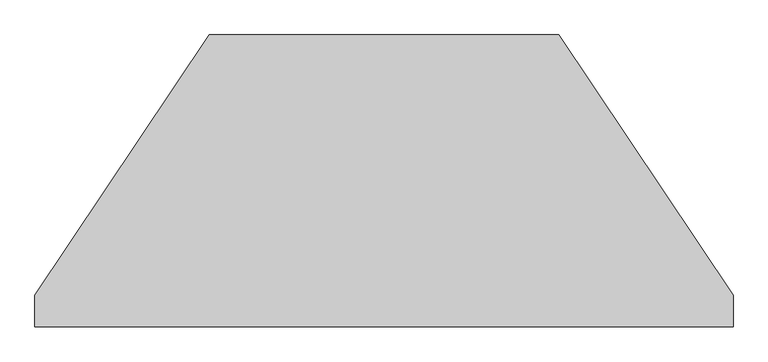
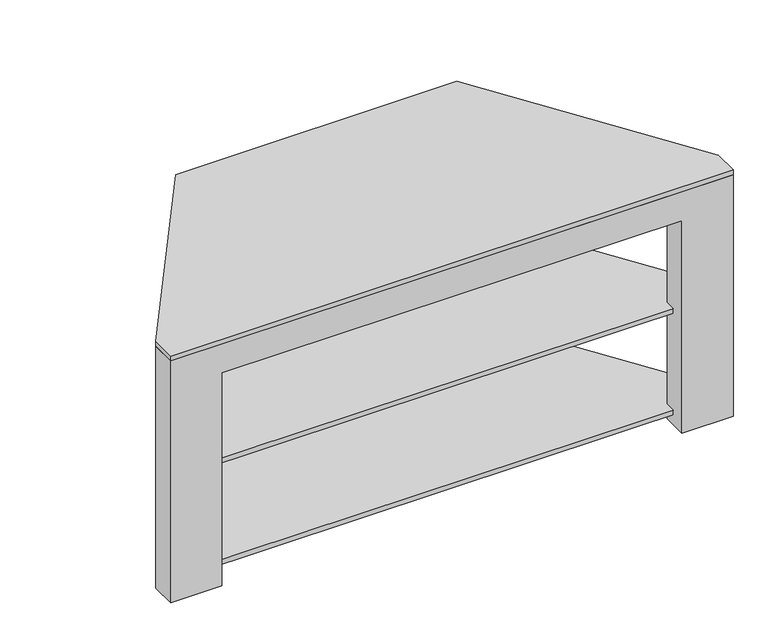
"""IFC4 building model written with IfcOpenShell, lengths in millimetres: furniture geometry."""

from ifc_helpers import new_model, si_unit, point, frame, frame_2d, origin, place, context, project, spatial, polyline, circle_curve, trimmed, segment, composite_curve, outline, extrude, faceted_brep, source, transform, mapped, element, save


def furniture_40ec15d9(model_context):
    return source(origin(), model_context, "Body", "SolidModel", [
        extrude(outline(polyline([(420.3099533, -30.0), (625.1880021, -335.4545455), (625.1880021, -430.0), (-374.8119979, -430.0), (-374.8119979, -335.4545455), (-169.9339492, -30.0), (420.3099533, -30.0)])), frame((0.0, 0.0, 20.0), z_axis=(0.0, 0.0, 1.0), x_axis=(1.0, 0.0, 0.0)), (0.0, 0.0, 1.0), 10.0),
        extrude(outline(polyline([(420.3099533, -30.0), (625.1880021, -335.4545455), (625.1880021, -430.0), (-374.8119979, -430.0), (-374.8119979, -335.4545455), (-169.9339492, -30.0), (420.3099533, -30.0)])), frame((0.0, 0.0, 230.0), z_axis=(0.0, 0.0, 1.0), x_axis=(1.0, 0.0, 0.0)), (0.0, 0.0, 1.0), 10.0),
        extrude(outline(polyline([(400.1880021, 0.0), (675.1880021, -410.0), (675.1880021, -460.0), (-424.8119979, -460.0), (-424.8119979, -410.0), (-149.8119979, 0.0), (400.1880021, 0.0)])), frame((0.0, 0.0, 500.0), z_axis=(0.0, 0.0, 1.0), x_axis=(1.0, 0.0, 0.0)), (0.0, 0.0, 1.0), 10.0),
        extrude(outline(polyline([(-50.0, 500.0), (0.0, 500.0), (0.0, 0.0), (-50.0, 0.0), (-50.0, 20.0), (-30.0, 20.0), (-30.0, 30.0), (-50.0, 30.0), (-50.0, 230.0), (-30.0, 230.0), (-30.0, 240.0), (-50.0, 240.0), (-50.0, 500.0)])), frame((-149.8119979, 0.0, 0.0), z_axis=(1.0, 0.0, 0.0), x_axis=(0.0, 1.0, 0.0)), (0.0, 0.0, 1.0), 100.0),
        extrude(outline(polyline([(-50.0, 500.0), (0.0, 500.0), (0.0, 0.0), (-50.0, 0.0), (-50.0, 20.0), (-30.0, 20.0), (-30.0, 30.0), (-50.0, 30.0), (-50.0, 230.0), (-30.0, 230.0), (-30.0, 240.0), (-50.0, 240.0), (-50.0, 500.0)])), frame((300.1880021, 0.0, 0.0), z_axis=(1.0, 0.0, 0.0), x_axis=(0.0, 1.0, 0.0)), (0.0, 0.0, 1.0), 100.0),
        faceted_brep([(-424.8119979, -460.0, 0.0), (-324.8119979, -460.0, 0.0), (-324.8119979, -460.0, 440.0), (575.1880021, -460.0, 440.0), (575.1880021, -460.0, 0.0), (675.1880021, -460.0, 0.0), (675.1880021, -460.0, 500.0), (-424.8119979, -460.0, 500.0), (-424.8119979, -410.0, 0.0), (-424.8119979, -410.0, 500.0), (675.1880021, -410.0, 500.0), (675.1880021, -410.0, 0.0), (575.1880021, -410.0, 0.0), (575.1880021, -410.0, 20.0), (625.1880021, -410.0, 20.0), (625.1880021, -410.0, 30.0), (575.1880021, -410.0, 30.0), (575.1880021, -410.0, 230.0), (625.1880021, -410.0, 230.0), (625.1880021, -410.0, 240.0), (575.1880021, -410.0, 240.0), (575.1880021, -410.0, 440.0), (-324.8119979, -410.0, 440.0), (-324.8119979, -410.0, 240.0), (-374.8119979, -410.0, 240.0), (-374.8119979, -410.0, 230.0), (-324.8119979, -410.0, 230.0), (-324.8119979, -410.0, 30.0), (-374.8119979, -410.0, 30.0), (-374.8119979, -410.0, 20.0), (-324.8119979, -410.0, 20.0), (-324.8119979, -410.0, 0.0), (-324.8119979, -430.0, 20.0), (-324.8119979, -430.0, 30.0), (-324.8119979, -430.0, 230.0), (-324.8119979, -430.0, 240.0), (575.1880021, -430.0, 240.0), (575.1880021, -430.0, 230.0), (575.1880021, -430.0, 30.0), (575.1880021, -430.0, 20.0), (625.1880021, -430.0, 240.0), (-374.8119979, -430.0, 240.0), (-374.8119979, -430.0, 230.0), (625.1880021, -430.0, 230.0), (625.1880021, -430.0, 30.0), (-374.8119979, -430.0, 30.0), (-374.8119979, -430.0, 20.0), (625.1880021, -430.0, 20.0)], [[[0, 1, 2, 3, 4, 5, 6, 7]], [[8, 9, 10, 11, 12, 13, 14, 15, 16, 17, 18, 19, 20, 21, 22, 23, 24, 25, 26, 27, 28, 29, 30, 31]], [[1, 0, 8, 31]], [[2, 1, 31, 30, 32, 33, 27, 26, 34, 35, 23, 22]], [[3, 2, 22, 21]], [[4, 3, 21, 20, 36, 37, 17, 16, 38, 39, 13, 12]], [[5, 4, 12, 11]], [[6, 5, 11, 10]], [[7, 6, 10, 9]], [[0, 7, 9, 8]], [[19, 40, 36, 20]], [[35, 41, 24, 23]], [[25, 42, 34, 26]], [[37, 43, 18, 17]], [[41, 42, 25, 24]], [[42, 41, 35, 34]], [[40, 43, 37, 36]], [[43, 40, 19, 18]], [[15, 44, 38, 16]], [[33, 45, 28, 27]], [[29, 46, 32, 30]], [[39, 47, 14, 13]], [[45, 46, 29, 28]], [[46, 45, 33, 32]], [[44, 47, 39, 38]], [[47, 44, 15, 14]]]),
        extrude(outline(polyline([(0.0, 300.1880021), (500.0, 300.1880021), (500.0, -49.8119979), (0.0, -49.8119979), (0.0, 300.1880021)]), holes=[composite_curve([segment(polyline([(245.0, 145.1700818), (245.0, 105.2059224)]), True, "CONTINUOUS"), segment(trimmed(circle_curve(frame_2d((257.5, 105.2059224)), 12.5), [point((245.0, 105.2059224))], [point((270.0, 105.2059224))], True, "CARTESIAN"), True, "CONTINUOUS"), segment(polyline([(270.0, 105.2059224), (270.0, 145.1700818)]), True, "CONTINUOUS"), segment(trimmed(circle_curve(frame_2d((257.5, 145.1700818)), 12.5), [point((270.0, 145.1700818))], [point((245.0, 145.1700818))], True, "CARTESIAN"), True, "CONTINUOUS")], self_intersect=False), composite_curve([segment(polyline([(35.0, 145.1880021), (35.0, 105.2059224)]), True, "CONTINUOUS"), segment(trimmed(circle_curve(frame_2d((47.5, 105.2059224)), 12.5), [point((35.0, 105.2059224))], [point((60.0, 105.2059224))], True, "CARTESIAN"), True, "CONTINUOUS"), segment(polyline([(60.0, 105.2059224), (60.0, 145.1880021)]), True, "CONTINUOUS"), segment(trimmed(circle_curve(frame_2d((47.5, 145.1880021)), 12.5), [point((60.0, 145.1880021))], [point((35.0, 145.1880021))], True, "CARTESIAN"), True, "CONTINUOUS")], self_intersect=False)]), frame((0.0, -30.0, 0.0), z_axis=(0.0, 1.0, 0.0), x_axis=(0.0, 0.0, 1.0)), (0.0, 0.0, 1.0), 10.0),
    ])


if __name__ == "__main__":
    model = new_model("IFC4")
    model_context = context("Model", 3, world=origin())
    ifc_project = project(units=[si_unit("LENGTHUNIT", "METRE", prefix="MILLI")], contexts=[model_context])
    site = spatial("IfcSite", under=ifc_project)
    building = spatial("IfcBuilding", under=site)
    placement = place(None, origin())
    furniture_shape = furniture_40ec15d9(model_context)
    element("IfcFurniture", 1, at=placement, inside=building, context=model_context, shape_type="MappedRepresentation", body=[
        mapped(furniture_shape, transform((0.0, 0.0, 0.0), x_axis=(1.0, 0.0, 0.0), y_axis=(0.0, 1.0, 0.0), z_axis=(0.0, 0.0, 1.0))),
    ])
    save(model, "model.ifc")

# Revit data of these elements
# Type
#   Depth = 1' - 6.11024"
#   Width = 3' - 7.30709"
#   Height = 1' - 7.68504"
#   Finish = Melamine - Gray
#   Default Elevation = 0
# Element 1 (IfcFurniture)
#   Materials on its faces: "Melamine - Gray", "Glass - Shelves"
# Materials
#   "Melamine - Gray": class "Wood", colour RGB 49 49 49, transparency 0
#   "Glass - Shelves": class "Glass", colour RGB 167 167 167, transparency 0.9
